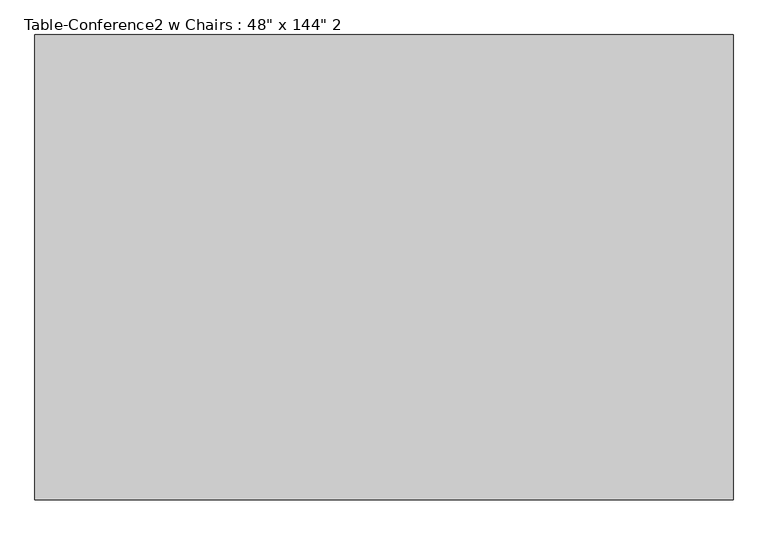
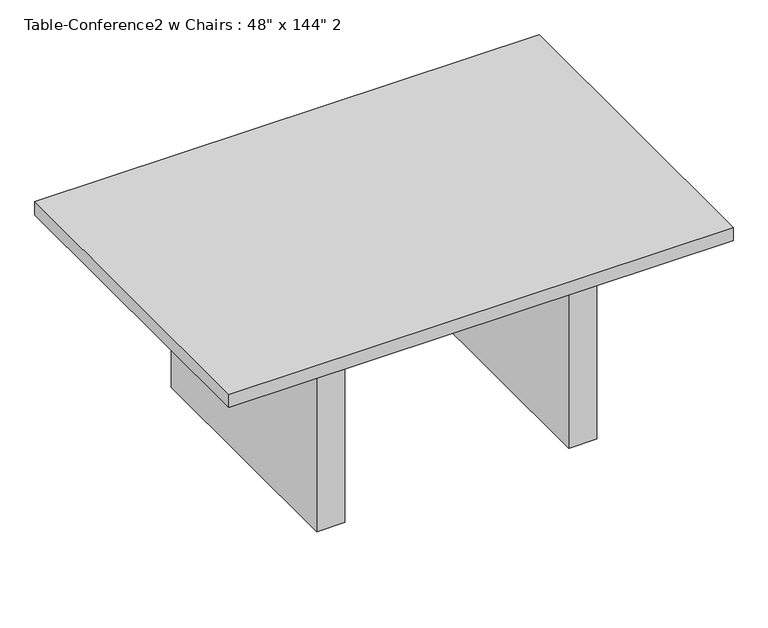
"""IFC4 building model written with IfcOpenShell, lengths in millimetres: furniture geometry."""

from ifc_helpers import new_model, si_unit, frame, origin, origin_with_axes, place, context, project, spatial, polyline, outline, extrude, source, transform, mapped, element, save


def furniture_0bcc43ae(model_context):
    return source(origin(), model_context, "Body", "SweptSolid", [
        extrude(outline(polyline([(914.4, -609.6), (-914.4, -609.6), (-914.4, 609.6), (914.4, 609.6), (914.4, -609.6)])), frame((0.0, 0.0, 711.2), z_axis=(0.0, 0.0, 1.0), x_axis=(1.0, 0.0, 0.0)), (0.0, 0.0, 1.0), 50.8),
        extrude(outline(polyline([(-406.4, -457.2), (-508.0, -457.2), (-508.0, 457.2), (-406.4, 457.2), (-406.4, -457.2)])), origin_with_axes(), (0.0, 0.0, 1.0), 711.2),
        extrude(outline(polyline([(508.0, -457.2), (406.4, -457.2), (406.4, 457.2), (508.0, 457.2), (508.0, -457.2)])), origin_with_axes(), (0.0, 0.0, 1.0), 711.2),
        extrude(outline(polyline([(406.4, 457.2), (406.4, 419.1), (-406.4, 419.1), (-406.4, 457.2), (406.4, 457.2)])), frame((0.0, 0.0, 609.6), z_axis=(0.0, 0.0, 1.0), x_axis=(1.0, 0.0, 0.0)), (0.0, 0.0, 1.0), 101.6),
        extrude(outline(polyline([(406.4, -457.2), (-406.4, -457.2), (-406.4, -419.1), (406.4, -419.1), (406.4, -457.2)])), frame((0.0, 0.0, 609.6), z_axis=(0.0, 0.0, 1.0), x_axis=(1.0, 0.0, 0.0)), (0.0, 0.0, 1.0), 101.6),
    ])


if __name__ == "__main__":
    model = new_model("IFC4")
    model_context = context("Model", 3, world=origin())
    ifc_project = project(units=[si_unit("LENGTHUNIT", "METRE", prefix="MILLI")], contexts=[model_context])
    site = spatial("IfcSite", under=ifc_project)
    building = spatial("IfcBuilding", under=site)
    placement = place(None, origin())
    furniture_shape = furniture_0bcc43ae(model_context)
    element("IfcFurniture", 1, ObjectType="Table-Conference2 w Chairs : 48\" x 144\" 2", at=placement, inside=building, context=model_context, shape_type="MappedRepresentation", body=[
        mapped(furniture_shape, transform((0.0, 0.0, 0.0), x_axis=(1.0, 0.0, 0.0), y_axis=(0.0, 1.0, 0.0), z_axis=(0.0, 0.0, 1.0))),
    ])
    save(model, "model.ifc")

# Revit data of these elements
# Type "Table-Conference2 w Chairs : 48\" x 144\" 2"
#   Assembly Code = "E2020200"
#   Description = "Seating 12-14"
#   Height = 2' - 6"
#   Length = 6' - 0"
#   Width = 4' - 0"
#   Number Of Chairs One Side = 2
#   Number Of Chairs = 6
#   Material = Wood - Cherry
#   Default Elevation = 0
# Element 1 (IfcFurniture, "Table-Conference2 w Chairs : 48\" x 144\" 2")
#   Materials on its faces: "Wood - Cherry"
# Materials
#   "Wood - Cherry": colour RGB 151 75 0, transparency 0
